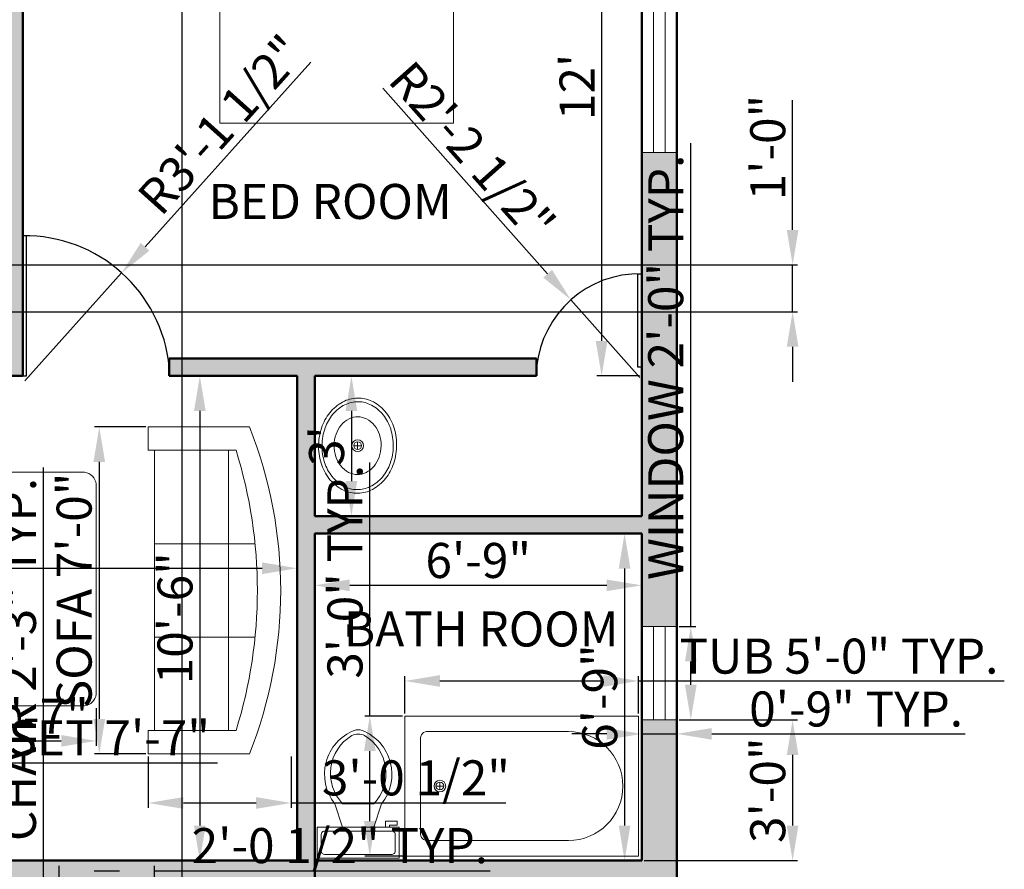
# Model space of a CAD drawing. Units: inches. Extents: x 875413 to 876020, y 447446 to 448210.
# Tile 7 of 8: x 875767 to 876020, y 447795 to 448013. Entities that reach past the tile are written whole.
import ezdxf

# ---------------------------------------------------------------- set-up
doc = ezdxf.new("R2010")
doc.units = ezdxf.units.IN
for name, color, linetype, lineweight in [('A-ANNO-DIMS', 2, 'Continuous', 13), ('A-AREA-IDEN', 7, 'Continuous', 25), ('A-DOOR', 3, 'Continuous', 25), ('A-FLOR-FIXT', 9, 'Continuous', 18), ('A-FURN', 8, 'Continuous', 18), ('A-GLAZ', 4, 'Continuous', 20), ('A-WALL', 7, 'Continuous', 50)]:
    doc.layers.add(name, color=color, linetype=linetype, lineweight=lineweight)
doc.layers.add('A-WALL-PATT', color=18, linetype='Continuous', lineweight=13, true_color=0x000000)
doc.styles.get("Standard").update_dxf_attribs({"font": 'arial.ttf'})
doc.dimstyles.new('ISO-25', dxfattribs={"dimtxt": 9, "dimasz": 9, "dimexe": 1.25, "dimexo": 0.625, "dimtad": 1, "dimdec": 1, "dimrnd": 9, "dimlunit": 3, "dimtxsty": 'Standard', "dimcen": 2.5, "dimadec": 0, "dimazin": 0, "dimtfac": 1, "dimtdec": 1, "dimtmove": 0, "dimatfit": 3, "dimfxl": 1, "dimarcsym": 0})

# ---------------------------------------------------------------- blocks, each defined once
blk = doc.blocks.new('*D6')
at = {"layer": 'A-ANNO-DIMS', "color": 0, "lineweight": -2, "transparency": 16777216}
for p, q in [((875926.08, 448070.02), (875915.14, 448070.02)), ((875916.39, 448061.02), (875916.39, 447930.52)), ((875926.08, 447921.52), (875915.14, 447921.52))]:
    blk.add_line(p, q, dxfattribs=at)
at = {"layer": 'A-ANNO-DIMS', "color": 0, "transparency": 16777216}
for points in [[(875914.89, 448061.02), (875917.89, 448061.02), (875916.39, 448070.02)], [(875914.89, 447930.52), (875917.89, 447930.52), (875916.39, 447921.52)]]:
    blk.add_solid(points, dxfattribs=at)
at = {"layer": 'Defpoints', "color": 0, "transparency": 16777216}
for p in [(875926.7, 448070.02), (875916.39, 447921.52), (875926.7, 447921.52)]:
    blk.add_point(p, dxfattribs=at)
at = {"layer": 'A-ANNO-DIMS', "color": 0, "transparency": 16777216, "insert": (875911.25, 447995.77), "char_height": 9, "attachment_point": 5, "rotation": 90}
blk.add_mtext("12'", dxfattribs=at)
blk = doc.blocks.new('*D10')
at = {"layer": 'A-ANNO-DIMS', "color": 0, "lineweight": -2, "transparency": 16777216}
for p, q in [((875843.33, 447921.52), (875853.37, 447921.52)), ((875852.12, 447912.52), (875852.12, 447894.52)), ((875843.33, 447885.52), (875853.37, 447885.52))]:
    blk.add_line(p, q, dxfattribs=at)
at = {"layer": 'A-ANNO-DIMS', "color": 0, "transparency": 16777216}
for points in [[(875850.62, 447912.52), (875853.62, 447912.52), (875852.12, 447921.52)], [(875850.62, 447894.52), (875853.62, 447894.52), (875852.12, 447885.52)]]:
    blk.add_solid(points, dxfattribs=at)
at = {"layer": 'Defpoints', "color": 0, "transparency": 16777216}
for p in [(875842.7, 447921.52), (875842.7, 447885.52), (875852.12, 447885.52)]:
    blk.add_point(p, dxfattribs=at)
at = {"layer": 'A-ANNO-DIMS', "color": 0, "transparency": 16777216, "insert": (875846.9, 447903.52), "char_height": 9, "attachment_point": 5, "rotation": 90}
blk.add_mtext("3'", dxfattribs=at)
blk = doc.blocks.new('*D11')
at = {"layer": 'A-ANNO-DIMS', "color": 0, "lineweight": -2, "transparency": 16777216}
for p, q in [((875842.7, 447880.39), (875842.7, 447866.47)), ((875926.7, 447880.39), (875926.7, 447866.47)), ((875917.7, 447867.72), (875851.7, 447867.72))]:
    blk.add_line(p, q, dxfattribs=at)
at = {"layer": 'A-ANNO-DIMS', "color": 0, "transparency": 16777216}
for points in [[(875851.7, 447869.22), (875851.7, 447866.22), (875842.7, 447867.72)], [(875917.7, 447869.22), (875917.7, 447866.22), (875926.7, 447867.72)]]:
    blk.add_solid(points, dxfattribs=at)
at = {"layer": 'Defpoints', "color": 0, "transparency": 16777216}
for p in [(875842.7, 447881.02), (875926.7, 447881.02), (875842.7, 447867.72)]:
    blk.add_point(p, dxfattribs=at)
at = {"layer": 'A-ANNO-DIMS', "color": 0, "transparency": 16777216, "insert": (875884.7, 447872.94), "char_height": 9, "attachment_point": 5}
blk.add_mtext('6\'-9"', dxfattribs=at)
blk = doc.blocks.new('*D12')
at = {"layer": 'A-ANNO-DIMS', "color": 0, "lineweight": -2, "transparency": 16777216}
for p, q in [((875926.08, 447881.02), (875921.04, 447881.02)), ((875922.29, 447872.02), (875922.29, 447806.02)), ((875926.08, 447797.02), (875921.04, 447797.02))]:
    blk.add_line(p, q, dxfattribs=at)
at = {"layer": 'A-ANNO-DIMS', "color": 0, "transparency": 16777216}
for points in [[(875920.79, 447872.02), (875923.79, 447872.02), (875922.29, 447881.02)], [(875920.79, 447806.02), (875923.79, 447806.02), (875922.29, 447797.02)]]:
    blk.add_solid(points, dxfattribs=at)
at = {"layer": 'Defpoints', "color": 0, "transparency": 16777216}
for p in [(875926.7, 447881.02), (875922.29, 447797.02), (875926.7, 447797.02)]:
    blk.add_point(p, dxfattribs=at)
at = {"layer": 'A-ANNO-DIMS', "color": 0, "transparency": 16777216, "insert": (875917.07, 447839.02), "char_height": 9, "attachment_point": 5, "rotation": 90}
blk.add_mtext('6\'-9"', dxfattribs=at)
blk = doc.blocks.new('*D13')
at = {"layer": 'A-ANNO-DIMS', "color": 0, "lineweight": -2, "transparency": 16777216}
for p, q in [((875571.2, 447920.89), (875571.2, 447870.86)), ((875838.2, 447920.89), (875838.2, 447870.86)), ((875580.2, 447872.11), (875829.2, 447872.11))]:
    blk.add_line(p, q, dxfattribs=at)
at = {"layer": 'A-ANNO-DIMS', "color": 0, "transparency": 16777216}
for points in [[(875580.2, 447873.61), (875580.2, 447870.61), (875571.2, 447872.11)], [(875829.2, 447873.61), (875829.2, 447870.61), (875838.2, 447872.11)]]:
    blk.add_solid(points, dxfattribs=at)
at = {"layer": 'Defpoints', "color": 0, "transparency": 16777216}
for p in [(875571.2, 447921.52), (875838.2, 447921.52), (875838.2, 447872.11)]:
    blk.add_point(p, dxfattribs=at)
at = {"layer": 'A-ANNO-DIMS', "color": 0, "transparency": 16777216, "insert": (875704.7, 447877.33), "char_height": 9, "attachment_point": 5}
blk.add_mtext('22\'-6"', dxfattribs=at)
blk = doc.blocks.new('*D14')
at = {"layer": 'A-ANNO-DIMS', "color": 0, "lineweight": -2, "transparency": 16777216}
for p, q in [((875837.58, 447921.52), (875811.94, 447921.52)), ((875813.19, 447912.52), (875813.19, 447806.02)), ((875837.58, 447797.02), (875811.94, 447797.02))]:
    blk.add_line(p, q, dxfattribs=at)
at = {"layer": 'A-ANNO-DIMS', "color": 0, "transparency": 16777216}
for points in [[(875811.69, 447912.52), (875814.69, 447912.52), (875813.19, 447921.52)], [(875811.69, 447806.02), (875814.69, 447806.02), (875813.19, 447797.02)]]:
    blk.add_solid(points, dxfattribs=at)
at = {"layer": 'Defpoints', "color": 0, "transparency": 16777216}
for p in [(875838.2, 447921.52), (875813.19, 447797.02), (875838.2, 447797.02)]:
    blk.add_point(p, dxfattribs=at)
at = {"layer": 'A-ANNO-DIMS', "color": 0, "transparency": 16777216, "insert": (875807.97, 447859.27), "char_height": 9, "attachment_point": 5, "rotation": 90}
blk.add_mtext('10\'-6"', dxfattribs=at)
blk = doc.blocks.new('Bed - Queen')
for p, q in [((0, -80.00003), (0, 0)), ((0, 0), (59.99999, 0)), ((59.99999, 0), (59.99999, -80.00003)), ((7.99999, -1.2), (28.79998, -1.2)), ((7.99999, -14.4), (7.99999, -1.2)), ((28.79998, -1.2), (28.79998, -14.4)), ((31.19999, -1.2), (51.99999, -1.2)), ((31.19999, -14.4), (31.19999, -1.2)), ((51.99999, -1.2), (51.99999, -16.4)), ((0, -14.4), (44.8, -14.4)), ((59.99999, -29.6), (44.8, -14.4)), ((44.8, -14.4), (44.8, -29.6)), ((44.8, -16.8), (0, -16.8)), ((51.99999, -16.4), (46.79936, -16.4)), ((44.8, -29.6), (59.99999, -29.6)), ((59.99999, -80.00003), (0, -80.00003))]:
    blk.add_line(p, q)
blk = doc.blocks.new('Sink - Oval top')
for p, q in [((-1, 0), (1, 0)), ((0, 1), (0, -1))]:
    blk.add_line(p, q)
for points in [[(-12.23, 0.39, 0.117634), (-11.46, -3.36, 0.104469), (-8.88, -6.8, 0.090016), (-5.08, -9.07, 0.08192), (-0.32, -10.02, 0.08192), (4.49, -9.38, 0.090016), (8.42, -7.36, 0.104469), (11.22, -4.09, 0.117634), (12.23, -0.39, 0.117634), (11.46, 3.36, 0.104469), (8.88, 6.8, 0.090016), (5.08, 9.07, 0.08192), (0.32, 10.02, 0.08192), (-4.49, 9.38, 0.090016), (-8.42, 7.36, 0.104469), (-11.22, 4.09, 0.117634)], [(-11.29, 0.16, 0.118622), (-10.52, -3.25, 0.104678), (-8.07, -6.36, 0.089562), (-4.54, -8.37, 0.081185), (-0.13, -9.15, 0.081185), (4.3, -8.49, 0.089562), (7.89, -6.58, 0.104678), (10.42, -3.55, 0.118622), (11.29, -0.16, 0.118622), (10.52, 3.25, 0.104678), (8.07, 6.36, 0.089562), (4.54, 8.37, 0.081185), (0.13, 9.15, 0.081185), (-4.3, 8.49, 0.089562), (-7.89, 6.58, 0.104678), (-10.42, 3.55, 0.118622)], [(-7.42, 0.08, 0.118283), (-6.91, -2.17, 0.104607), (-5.29, -4.21, 0.089718), (-2.97, -5.53, 0.081436), (-0.07, -6.04, 0.081436), (2.84, -5.59, 0.089718), (5.2, -4.33, 0.104607), (6.86, -2.32, 0.118283), (7.42, -0.08, 0.118283), (6.91, 2.17, 0.104607), (5.29, 4.21, 0.089718), (2.97, 5.53, 0.081436), (0.07, 6.04, 0.081436), (-2.84, 5.59, 0.089718), (-5.2, 4.33, 0.104607), (-6.86, 2.32, 0.118283)]]:
    blk.add_lwpolyline(points, format="xyb", close=True)
for radius in [1.5, 1]:
    blk.add_circle((0, 0), radius)
blk = doc.blocks.new('Toilet - top')
for p, q in [((9.5, -6), (9.5, -2)), ((-10, -8.5), (-8, -8.5)), ((-10, -9.5), (-10, -8.5)), ((-7, -9.5), (-10, -9.5)), ((-8, -8.5), (-8, -8)), ((-7, -8), (-7, -9.5)), ((-4, -8), (-6, -14)), ((4, -8), (6, -14)), ((4, -14), (-4, -14))]:
    blk.add_line(p, q)
blk.add_lwpolyline([(10.5, -8), (10.5, 0), (-10.5, 0), (-10.5, -8)], close=True)
for points in [[(-9.5, -2), (-9.5, -6)], [(8.5, -1), (-8.5, -1)], [(-8.5, -7), (8.5, -7)]]:
    blk.add_lwpolyline(points)
for centre, radius, start, end in [((-8.62, -1.88), 0.884, 81.8699, 188.1301), ((8.62, -1.88), 0.884, 351.8699, 98.1301), ((-8.62, -6.12), 0.884, 171.8699, 278.1301), ((8.62, -6.12), 0.884, 261.8699, 8.1301), ((3.52, -21.58), 12.17, 141.4691, 247.9714), ((4.2, -21.82), 11.33, 136.3677, 238.9468), ((-3.52, -21.58), 12.17, 292.0284, 38.5307), ((-4.2, -21.82), 11.33, 301.053, 43.6321), ((0, -27.88), 4, 245.7318, 294.2682), ((0, -29), 4, 254.8605, 285.1395)]:
    blk.add_arc(centre, radius, start, end)
blk = doc.blocks.new('Sofa - Roundback 7 ft.')
for p, q in [((-12.00002, -32.4421), (-12.00003, -6.5971)), ((11.99997, -32.4421), (11.99998, -6.5971)), ((-36.000027, -34), (-36.000027, -11.4696)), ((35.99998, -34), (35.99998, -11.4696)), ((-35.999844, -13.3819), (35.9998, -13.3819)), ((-36.000027, -32.4421), (35.99998, -32.4421))]:
    blk.add_line(p, q)
for points in [[(-36.000027, -34), (-42.000027, -34), (-42.000027, -8)], [(41.99998, -8), (41.99998, -34), (35.99998, -34)]]:
    blk.add_lwpolyline(points)
for centre, radius, start, end in [((0, -114.25), 114.25, 68.43141, 111.5686), ((-0.00001, -127.1968), 121.1968, 72.72033, 107.2797)]:
    blk.add_arc(centre, radius, start, end)
blk = doc.blocks.new('Desk - 30 x 60 in.')
for p, q in [((-26.999995, 0), (26.999995, 0)), ((-29.999995, -27), (-29.999995, -3)), ((29.999995, -3), (29.999995, -27)), ((26.999995, -30), (-26.999995, -30)), ((-20.000005, -30), (-20.000005, -31)), ((-16.000005, -31), (-16.000005, -30)), ((15.999995, -31), (15.999995, -30)), ((19.999995, -30), (19.999995, -31)), ((-20.000005, -31), (-16.000005, -31)), ((19.999995, -31), (15.999995, -31))]:
    blk.add_line(p, q)
for centre, start, end in [((-26.499995, -3.5), 98.1301, 171.8699), ((26.499995, -3.5), 8.130102, 81.8699), ((-26.499995, -26.5), 188.1301, 261.8699), ((26.499995, -26.5), 278.1301, 351.8699)]:
    blk.add_arc(centre, 3.535534, start, end)
blk = doc.blocks.new('Bath Tub - 26 x 60 in.')
for p, q in [((9, -17), (9, -19)), ((8, -18), (10, -18))]:
    blk.add_line(p, q)
blk.add_lwpolyline([(0, -36), (0, 0), (60, 0), (60, -36)], close=True)
for points in [[(6, -4), (42, -4)], [(4, -30), (4, -6)], [(42, -32), (6, -32)]]:
    blk.add_lwpolyline(points)
for radius in [1.5, 1]:
    blk.add_circle((9, -18), radius)
for centre, radius, start, end in [((5.75, -5.75), 1.77, 81.8699, 188.1301), ((42, -18), 14, 270, 90), ((5.75, -30.25), 1.77, 171.8699, 278.1301)]:
    blk.add_arc(centre, radius, start, end)
blk = doc.blocks.new('WIN-60IN')
for p, q in [((0, 9), (0, 0)), ((60, 9), (60, 0)), ((60, 6), (0, 6)), ((60, 3), (0, 3))]:
    blk.add_line(p, q)
blk = doc.blocks.new('WIN-24IN')
for p, q in [((0, 24), (9, 24)), ((3, 0), (3, 24)), ((6, 0), (6, 24)), ((0, 0), (9, 0))]:
    blk.add_line(p, q)
blk = doc.blocks.new('*D43')
at = {"layer": 'A-ANNO-DIMS', "color": 0, "lineweight": -2, "transparency": 16777216}
for p, q in [((875939.3, 447857.16), (875939.3, 447981.3)), ((875936.33, 447857.16), (875940.55, 447857.16)), ((875939.3, 447842.16), (875939.3, 447848.16)), ((875936.33, 447833.16), (875940.55, 447833.16))]:
    blk.add_line(p, q, dxfattribs=at)
at = {"layer": 'A-ANNO-DIMS', "color": 0, "transparency": 16777216}
for points in [[(875937.8, 447848.16), (875940.8, 447848.16), (875939.3, 447857.16)], [(875937.8, 447842.16), (875940.8, 447842.16), (875939.3, 447833.16)]]:
    blk.add_solid(points, dxfattribs=at)
at = {"layer": 'Defpoints', "color": 0, "transparency": 16777216}
for p in [(875935.7, 447857.16), (875939.3, 447857.16), (875935.7, 447833.16)]:
    blk.add_point(p, dxfattribs=at)
at = {"layer": 'A-ANNO-DIMS', "color": 0, "transparency": 16777216, "insert": (875934.02, 447923.73), "char_height": 9, "attachment_point": 5, "rotation": 90}
blk.add_mtext('WINDOW 2\'-0" TYP.', dxfattribs=at)
blk = doc.blocks.new('*D44')
at = {"layer": 'A-ANNO-DIMS', "color": 0, "lineweight": -2, "transparency": 16777216}
for p, q in [((875926.7, 447832.54), (875926.7, 447828.31)), ((875935.7, 447832.54), (875935.7, 447828.31)), ((875917.7, 447829.56), (875908.7, 447829.56)), ((875926.7, 447829.56), (875935.7, 447829.56)), ((875944.7, 447829.56), (876009.81, 447829.56))]:
    blk.add_line(p, q, dxfattribs=at)
at = {"layer": 'A-ANNO-DIMS', "color": 0, "transparency": 16777216}
for points in [[(875917.7, 447831.06), (875917.7, 447828.06), (875926.7, 447829.56)], [(875944.7, 447831.06), (875944.7, 447828.06), (875935.7, 447829.56)]]:
    blk.add_solid(points, dxfattribs=at)
at = {"layer": 'Defpoints', "color": 0, "transparency": 16777216}
for p in [(875926.7, 447833.16), (875935.7, 447833.16), (875935.7, 447829.56)]:
    blk.add_point(p, dxfattribs=at)
at = {"layer": 'A-ANNO-DIMS', "color": 0, "transparency": 16777216, "insert": (875981.76, 447834.78), "char_height": 9, "attachment_point": 5}
blk.add_mtext('0\'-9" TYP.', dxfattribs=at)
blk = doc.blocks.new('*D51')
at = {"layer": 'A-ANNO-DIMS', "color": 0, "lineweight": -2, "transparency": 16777216}
for p, q in [((875865.85, 447834.78), (875865.85, 447844.4)), ((875874.85, 447843.15), (875916.85, 447843.15)), ((875925.85, 447834.78), (875925.85, 447844.4)), ((875925.85, 447843.15), (876019.83, 447843.15))]:
    blk.add_line(p, q, dxfattribs=at)
at = {"layer": 'A-ANNO-DIMS', "color": 0, "transparency": 16777216}
for points in [[(875874.85, 447844.65), (875874.85, 447841.65), (875865.85, 447843.15)], [(875916.85, 447844.65), (875916.85, 447841.65), (875925.85, 447843.15)]]:
    blk.add_solid(points, dxfattribs=at)
at = {"layer": 'Defpoints', "color": 0, "transparency": 16777216}
for p in [(875925.85, 447843.15), (875865.85, 447834.15), (875925.85, 447834.15)]:
    blk.add_point(p, dxfattribs=at)
at = {"layer": 'A-ANNO-DIMS', "color": 0, "transparency": 16777216, "insert": (875977.34, 447848.37), "char_height": 9, "attachment_point": 5}
blk.add_mtext('TUB 5\'-0" TYP.', dxfattribs=at)
blk = doc.blocks.new('*D52')
at = {"layer": 'A-ANNO-DIMS', "color": 0, "lineweight": -2, "transparency": 16777216}
for p, q in [((875856.85, 447834.15), (875856.85, 447899.26)), ((875865.23, 447834.15), (875855.6, 447834.15)), ((875856.85, 447807.15), (875856.85, 447825.15)), ((875865.23, 447798.15), (875855.6, 447798.15))]:
    blk.add_line(p, q, dxfattribs=at)
at = {"layer": 'A-ANNO-DIMS', "color": 0, "transparency": 16777216}
for points in [[(875855.35, 447825.15), (875858.35, 447825.15), (875856.85, 447834.15)], [(875855.35, 447807.15), (875858.35, 447807.15), (875856.85, 447798.15)]]:
    blk.add_solid(points, dxfattribs=at)
at = {"layer": 'Defpoints', "color": 0, "transparency": 16777216}
for p in [(875856.85, 447834.15), (875865.85, 447834.15), (875865.85, 447798.15)]:
    blk.add_point(p, dxfattribs=at)
at = {"layer": 'A-ANNO-DIMS', "color": 0, "transparency": 16777216, "insert": (875851.63, 447871.2), "char_height": 9, "attachment_point": 5, "rotation": 90}
blk.add_mtext('3\'-0" TYP.', dxfattribs=at)
blk = doc.blocks.new('*D53')
at = {"layer": 'A-ANNO-DIMS', "color": 0, "lineweight": -2, "transparency": 16777216}
for p, q in [((875617.53, 447835.12), (875617.53, 447820.85)), ((875708.53, 447835.12), (875708.53, 447820.85)), ((875626.53, 447822.1), (875699.53, 447822.1)), ((875708.53, 447822.1), (875817.7, 447822.1))]:
    blk.add_line(p, q, dxfattribs=at)
at = {"layer": 'A-ANNO-DIMS', "color": 0, "transparency": 16777216}
for points in [[(875626.53, 447823.6), (875626.53, 447820.6), (875617.53, 447822.1)], [(875699.53, 447823.6), (875699.53, 447820.6), (875708.53, 447822.1)]]:
    blk.add_solid(points, dxfattribs=at)
at = {"layer": 'Defpoints', "color": 0, "transparency": 16777216}
for p in [(875617.53, 447835.75), (875708.53, 447835.75), (875708.53, 447822.1)]:
    blk.add_point(p, dxfattribs=at)
at = {"layer": 'A-ANNO-DIMS', "color": 0, "transparency": 16777216, "insert": (875767.62, 447827.38), "char_height": 9, "attachment_point": 5}
blk.add_mtext('DINING SET 7\'-7"', dxfattribs=at)
blk = doc.blocks.new('*D57')
at = {"layer": 'A-ANNO-DIMS', "color": 0, "lineweight": -2, "transparency": 16777216}
for p, q in [((875773.04, 447790.36), (875773.04, 447897.98)), ((875776.46, 447790.36), (875771.79, 447790.36)), ((875773.04, 447772.36), (875773.04, 447781.36)), ((875776.46, 447763.36), (875771.79, 447763.36))]:
    blk.add_line(p, q, dxfattribs=at)
at = {"layer": 'A-ANNO-DIMS', "color": 0, "transparency": 16777216}
for points in [[(875771.54, 447781.36), (875774.54, 447781.36), (875773.04, 447790.36)], [(875771.54, 447772.36), (875774.54, 447772.36), (875773.04, 447763.36)]]:
    blk.add_solid(points, dxfattribs=at)
at = {"layer": 'Defpoints', "color": 0, "transparency": 16777216}
for p in [(875773.04, 447790.36), (875777.09, 447790.36), (875777.09, 447763.36)]:
    blk.add_point(p, dxfattribs=at)
at = {"layer": 'A-ANNO-DIMS', "color": 0, "transparency": 16777216, "insert": (875767.76, 447848.67), "char_height": 9, "attachment_point": 5, "rotation": 90}
blk.add_mtext('CHAIR 2\'-3" TYP.', dxfattribs=at)
blk = doc.blocks.new('*D58')
at = {"layer": 'A-ANNO-DIMS', "color": 0, "lineweight": -2, "transparency": 16777216}
for p, q in [((875777.09, 447790.98), (875777.09, 447795.66)), ((875801.52, 447790.98), (875801.52, 447795.66)), ((875786.09, 447794.41), (875792.52, 447794.41)), ((875801.52, 447794.41), (875887.76, 447794.41))]:
    blk.add_line(p, q, dxfattribs=at)
at = {"layer": 'A-ANNO-DIMS', "color": 0, "transparency": 16777216}
for points in [[(875786.09, 447795.91), (875786.09, 447792.91), (875777.09, 447794.41)], [(875792.52, 447795.91), (875792.52, 447792.91), (875801.52, 447794.41)]]:
    blk.add_solid(points, dxfattribs=at)
at = {"layer": 'Defpoints', "color": 0, "transparency": 16777216}
for p in [(875801.52, 447794.41), (875777.09, 447790.36), (875801.52, 447790.36)]:
    blk.add_point(p, dxfattribs=at)
at = {"layer": 'A-ANNO-DIMS', "color": 0, "transparency": 16777216, "insert": (875849.14, 447799.69), "char_height": 9, "attachment_point": 5}
blk.add_mtext('2\'-0 1/2" TYP.', dxfattribs=at)
blk = doc.blocks.new('*D59')
at = {"layer": 'A-ANNO-DIMS', "color": 0, "lineweight": -2, "transparency": 16777216}
for p, q in [((875799.33, 447908.41), (875786.11, 447908.41)), ((875787.36, 447899.41), (875787.36, 447833.41)), ((875799.33, 447824.41), (875786.11, 447824.41))]:
    blk.add_line(p, q, dxfattribs=at)
at = {"layer": 'A-ANNO-DIMS', "color": 0, "transparency": 16777216}
for points in [[(875785.86, 447899.41), (875788.86, 447899.41), (875787.36, 447908.41)], [(875785.86, 447833.41), (875788.86, 447833.41), (875787.36, 447824.41)]]:
    blk.add_solid(points, dxfattribs=at)
at = {"layer": 'Defpoints', "color": 0, "transparency": 16777216}
for p in [(875799.96, 447908.41), (875787.36, 447824.41), (875799.96, 447824.41)]:
    blk.add_point(p, dxfattribs=at)
at = {"layer": 'A-ANNO-DIMS', "color": 0, "transparency": 16777216, "insert": (875782.07, 447866.41), "char_height": 9, "attachment_point": 5, "rotation": 90}
blk.add_mtext('SOFA 7\'-0"', dxfattribs=at)
blk = doc.blocks.new('*D60')
at = {"layer": 'A-ANNO-DIMS', "color": 0, "lineweight": -2, "transparency": 16777216}
for p, q in [((875799.96, 447823.78), (875799.96, 447810.56)), ((875836.62, 447823.78), (875836.62, 447810.56)), ((875808.96, 447811.81), (875827.62, 447811.81)), ((875836.62, 447811.81), (875891.76, 447811.81))]:
    blk.add_line(p, q, dxfattribs=at)
at = {"layer": 'A-ANNO-DIMS', "color": 0, "transparency": 16777216}
for points in [[(875808.96, 447813.31), (875808.96, 447810.31), (875799.96, 447811.81)], [(875827.62, 447813.31), (875827.62, 447810.31), (875836.62, 447811.81)]]:
    blk.add_solid(points, dxfattribs=at)
at = {"layer": 'Defpoints', "color": 0, "transparency": 16777216}
for p in [(875799.96, 447824.41), (875836.62, 447824.41), (875836.62, 447811.81)]:
    blk.add_point(p, dxfattribs=at)
at = {"layer": 'A-ANNO-DIMS', "color": 0, "transparency": 16777216, "insert": (875868.69, 447817.09), "char_height": 9, "attachment_point": 5}
blk.add_mtext('3\'-0 1/2"', dxfattribs=at)
blk = doc.blocks.new('*D62')
at = {"layer": 'A-ANNO-DIMS', "color": 0, "lineweight": -2, "transparency": 16777216}
for p, q in [((875755.58, 447836.14), (875755.58, 447826.52)), ((875786.58, 447836.14), (875786.58, 447826.52)), ((875764.58, 447827.77), (875777.58, 447827.77))]:
    blk.add_line(p, q, dxfattribs=at)
at = {"layer": 'A-ANNO-DIMS', "color": 0, "transparency": 16777216}
for points in [[(875764.58, 447829.27), (875764.58, 447826.27), (875755.58, 447827.77)], [(875777.58, 447829.27), (875777.58, 447826.27), (875786.58, 447827.77)]]:
    blk.add_solid(points, dxfattribs=at)
at = {"layer": 'Defpoints', "color": 0, "transparency": 16777216}
for p in [(875755.58, 447836.77), (875786.58, 447836.77), (875786.58, 447827.77)]:
    blk.add_point(p, dxfattribs=at)
at = {"layer": 'A-ANNO-DIMS', "color": 0, "transparency": 16777216, "insert": (875771.08, 447832.91), "char_height": 9, "attachment_point": 5}
blk.add_mtext('2\'-7"', dxfattribs=at)
blk = doc.blocks.new('*D75')
at = {"layer": 'A-ANNO-DIMS', "color": 0, "lineweight": -2, "transparency": 16777216}
for p, q in [((875936.33, 447833.16), (875966.7, 447833.16)), ((875965.45, 447824.16), (875965.45, 447806.02)), ((875927.33, 447797.02), (875966.7, 447797.02))]:
    blk.add_line(p, q, dxfattribs=at)
at = {"layer": 'A-ANNO-DIMS', "color": 0, "transparency": 16777216}
for points in [[(875963.95, 447824.16), (875966.95, 447824.16), (875965.45, 447833.16)], [(875963.95, 447806.02), (875966.95, 447806.02), (875965.45, 447797.02)]]:
    blk.add_solid(points, dxfattribs=at)
at = {"layer": 'Defpoints', "color": 0, "transparency": 16777216}
for p in [(875935.7, 447833.16), (875926.7, 447797.02), (875965.45, 447797.02)]:
    blk.add_point(p, dxfattribs=at)
at = {"layer": 'A-ANNO-DIMS', "color": 0, "transparency": 16777216, "insert": (875960.23, 447815.09), "char_height": 9, "attachment_point": 5, "rotation": 90}
blk.add_mtext('3\'-0"', dxfattribs=at)
blk = doc.blocks.new('*D78')
at = {"layer": 'A-ANNO-DIMS', "color": 0, "lineweight": -2, "transparency": 16777216}
for p, q in [((875965.45, 447959.02), (875965.45, 447992.34)), ((875763.83, 447950.02), (875966.7, 447950.02)), ((875965.45, 447938.02), (875965.45, 447950.02)), ((875763.83, 447938.02), (875966.7, 447938.02)), ((875965.45, 447929.02), (875965.45, 447920.02))]:
    blk.add_line(p, q, dxfattribs=at)
at = {"layer": 'A-ANNO-DIMS', "color": 0, "transparency": 16777216}
for points in [[(875963.95, 447959.02), (875966.95, 447959.02), (875965.45, 447950.02)], [(875963.95, 447929.02), (875966.95, 447929.02), (875965.45, 447938.02)]]:
    blk.add_solid(points, dxfattribs=at)
at = {"layer": 'Defpoints', "color": 0, "transparency": 16777216}
for p in [(875763.2, 447950.02), (875965.45, 447950.02), (875763.2, 447938.02)]:
    blk.add_point(p, dxfattribs=at)
at = {"layer": 'A-ANNO-DIMS', "color": 0, "transparency": 16777216, "insert": (875960.23, 447980.18), "char_height": 9, "attachment_point": 5, "rotation": 90}
blk.add_mtext('1\'-0"', dxfattribs=at)
blk = doc.blocks.new('*D80')
at = {"layer": 'A-ANNO-DIMS', "color": 0, "lineweight": -2, "transparency": 16777216}
for p, q in [((875748.63, 447673.14), (875748.63, 448110.02)), ((875757.63, 448108.77), (875799.63, 448108.77)), ((875808.63, 447673.14), (875808.63, 448110.02))]:
    blk.add_line(p, q, dxfattribs=at)
at = {"layer": 'A-ANNO-DIMS', "color": 0, "transparency": 16777216}
for points in [[(875757.63, 448110.27), (875757.63, 448107.27), (875748.63, 448108.77)], [(875799.63, 448110.27), (875799.63, 448107.27), (875808.63, 448108.77)]]:
    blk.add_solid(points, dxfattribs=at)
at = {"layer": 'Defpoints', "color": 0, "transparency": 16777216}
for p in [(875808.63, 448108.77), (875748.63, 447672.52), (875808.63, 447672.52)]:
    blk.add_point(p, dxfattribs=at)
at = {"layer": 'A-ANNO-DIMS', "color": 0, "transparency": 16777216, "insert": (875778.63, 448113.99), "char_height": 9, "attachment_point": 5}
blk.add_mtext('5\'-0"', dxfattribs=at)
blk = doc.blocks.new('*D94')
at = {"layer": 'A-ANNO-DIMS', "color": 0, "lineweight": -2, "transparency": 16777216}
for p, q in [((875841.68, 448002.16), (875799.12, 447954.69)), ((875768.2, 447920.22), (875793.11, 447947.99))]:
    blk.add_line(p, q, dxfattribs=at)
at = {"layer": 'A-ANNO-DIMS', "color": 0, "transparency": 16777216}
blk.add_solid([(875798, 447955.69), (875800.23, 447953.69), (875793.11, 447947.99)], dxfattribs=at)
at = {"layer": 'Defpoints', "color": 0, "transparency": 16777216}
for p in [(875793.11, 447947.99), (875768.2, 447920.22)]:
    blk.add_point(p, dxfattribs=at)
at = {"layer": 'A-ANNO-DIMS', "color": 0, "transparency": 16777216, "insert": (875819.47, 447985.3), "char_height": 9, "attachment_point": 5, "rotation": 48.1157}
blk.add_mtext('R3\'-1 1/2"', dxfattribs=at)
blk = doc.blocks.new('*D100')
at = {"layer": 'A-ANNO-DIMS', "color": 0, "lineweight": -2, "transparency": 16777216}
for p, q in [((875860.18, 447995.43), (875902.53, 447947.77)), ((875926.2, 447921.14), (875908.51, 447941.05))]:
    blk.add_line(p, q, dxfattribs=at)
at = {"layer": 'A-ANNO-DIMS', "color": 0, "transparency": 16777216}
blk.add_solid([(875903.65, 447948.77), (875901.41, 447946.78), (875908.51, 447941.05)], dxfattribs=at)
at = {"layer": 'Defpoints', "color": 0, "transparency": 16777216}
for p in [(875908.51, 447941.05), (875926.2, 447921.14)]:
    blk.add_point(p, dxfattribs=at)
at = {"layer": 'A-ANNO-DIMS', "color": 0, "transparency": 16777216, "insert": (875882.31, 447978.47), "char_height": 9, "attachment_point": 5, "rotation": 311.6278}
blk.add_mtext('R2\'-2 1/2"', dxfattribs=at)

msp = doc.modelspace()

# ---------------------------------------------------------------- hatches: boundary and pattern name
at = {"layer": 'A-WALL-PATT'}
h = msp.add_hatch(color=256, dxfattribs=at)
h.dxf.hatch_style = 1
h.paths.add_polyline_path([(875470.7, 447985.13), (875461.7, 447985.13), (875461.7, 447865.29), (875470.7, 447865.29), (875470.7, 447881.02), (875566.7, 447881.02), (875566.7, 447797.02), (875571.2, 447797.02), (875571.2, 447885.52), (875571.2, 447921.52), (875603.29, 447921.52), (875603.29, 447926.02), (875501.27, 447926.02), (875501.27, 447921.52), (875566.7, 447921.52), (875566.7, 447885.52), (875470.7, 447885.52), (875470.7, 447921.52), (875470.7, 447926.02)])
h.paths.add_polyline_path([(875470.7, 448070.02), (875518.96, 448070.02), (875518.96, 448079.02), (875461.7, 448079.02), (875461.7, 448045.13), (875470.7, 448045.13)])
h.paths.add_polyline_path([(875819.9, 448079.02), (875578.96, 448079.02), (875578.96, 448070.02), (875638.7, 448070.02), (875638.7, 447921.52), (875643.2, 447921.52), (875643.2, 448070.02), (875763.2, 448070.02), (875763.2, 447921.52), (875767.7, 447921.52), (875767.7, 448070.02), (875819.9, 448070.02)])
h.paths.add_polyline_path([(875935.7, 447978.92), (875926.7, 447978.92), (875926.7, 447926.02), (875926.7, 447921.52), (875926.7, 447885.52), (875842.7, 447885.52), (875842.7, 447921.52), (875899.7, 447921.52), (875899.7, 447926.02), (875805.34, 447926.02), (875805.34, 447921.52), (875838.2, 447921.52), (875838.2, 447885.52), (875838.2, 447797.02), (875689.7, 447797.02), (875689.7, 447792.52), (875842.7, 447792.52), (875842.7, 447881.02), (875926.7, 447881.02), (875926.7, 447857.16), (875935.7, 447857.16)])
h.paths.add_polyline_path([(875935.7, 448079.02), (875879.9, 448079.02), (875879.9, 448070.02), (875926.7, 448070.02), (875926.7, 448038.92), (875935.7, 448038.92)])
h.paths.add_polyline_path([(875935.7, 447833.16), (875926.7, 447833.16), (875926.7, 447797.02), (875842.7, 447797.02), (875842.7, 447792.52), (875926.7, 447792.52), (875926.7, 447756.52), (875935.7, 447756.52)])
h.paths.add_polyline_path([(875935.7, 447732.52), (875926.7, 447732.52), (875926.7, 447692.75, -0.007222), (875926.81, 447692.41, -0.08192), (875927.45, 447687.6, -0.071798), (875926.7, 447683.4), (875926.7, 447672.52), (875808.63, 447672.52), (875808.63, 447668.02), (875926.7, 447668.02), (875926.7, 447663.19), (875935.7, 447663.19)])
h.paths.add_polyline_path([(875842.7, 447792.52), (875838.2, 447792.52), (875838.2, 447704.02), (875842.7, 447704.02)])
h.paths.add_polyline_path([(875470.7, 447792.52), (875619.2, 447792.52), (875619.2, 447797.02), (875470.7, 447797.02), (875470.7, 447841.29), (875461.7, 447841.29), (875461.7, 447764.71), (875470.7, 447764.71)])
h.paths.add_polyline_path([(875619.2, 447760.51), (875616.95, 447760.51, -0.018388), (875614.7, 447760.37), (875614.7, 447672.52), (875470.7, 447672.52), (875470.7, 447704.71), (875461.7, 447704.71), (875461.7, 447640.7), (875470.7, 447640.7), (875470.7, 447668.02), (875619.2, 447668.02)])
h.paths.add_polyline_path([(875511.12, 447554.02), (875470.7, 447554.02), (875470.7, 447580.7), (875461.7, 447580.7), (875461.7, 447545.02), (875511.12, 447545.02)])
h.paths.add_polyline_path([(875656.47, 447554.02), (875620.05, 447554.02, -0.057036), (875616.67, 447553.74, -0.040891), (875614.26, 447554.02), (875571.12, 447554.02), (875571.12, 447545.02), (875656.47, 447545.02)])
h.paths.add_polyline_path([(875643.2, 447613.27), (875685.21, 447613.27), (875685.21, 447617.77), (875685.21, 447623.8), (875680.71, 447623.8), (875680.71, 447617.77), (875618.23, 447617.77), (875618.23, 447623.8), (875613.73, 447623.8), (875613.73, 447617.77), (875613.73, 447613.27), (875638.7, 447613.27), (875638.7, 447554.02), (875643.2, 447554.02)])
h.paths.add_polyline_path([(875694.2, 447760.28), (875689.7, 447760.28), (875689.7, 447668.02), (875748.63, 447668.02), (875748.63, 447672.52), (875694.2, 447672.52)])

# ---------------------------------------------------------------- linework, layer by layer
at = {"layer": 'A-DOOR'}
for p, q in [((875768.7, 447957.52), (875767.7, 447957.52)), ((875768.7, 447921.52), (875768.7, 447957.52)), ((875925.7, 447923.77), (875925.7, 447947.77)), ((875925.7, 447947.77), (875926.7, 447947.77)), ((875926.7, 447923.77), (875925.7, 447923.77)), ((875767.7, 447921.52), (875768.7, 447921.52))]:
    msp.add_line(p, q, dxfattribs=at)
for centre, radius, start, end in [((875768.2, 447920.22), 37.31, 5.4633, 90.768), ((875926.2, 447921.14), 26.64, 88.9244, 174.3318)]:
    msp.add_arc(centre, radius, start, end, dxfattribs=at)
at = {"layer": 'A-WALL'}
for p, q in [((875935.7, 447663.19), (875935.7, 448079.02)), ((875767.7, 448070.02), (875767.7, 447921.52)), ((875926.7, 447926.02), (875926.7, 448070.02)), ((875899.7, 447926.02), (875805.34, 447926.02)), ((875805.34, 447926.02), (875805.34, 447921.52)), ((875899.7, 447926.02), (875899.7, 447921.52)), ((875926.7, 447926.02), (875926.7, 447921.52)), ((875763.2, 447921.52), (875767.7, 447921.52)), ((875838.2, 447921.52), (875805.34, 447921.52)), ((875838.2, 447885.52), (875838.2, 447921.52)), ((875899.7, 447921.52), (875842.7, 447921.52)), ((875842.7, 447885.52), (875842.7, 447921.52)), ((875926.7, 447885.52), (875926.7, 447921.52)), ((875838.2, 447797.02), (875838.2, 447885.52)), ((875926.7, 447885.52), (875842.7, 447885.52)), ((875926.7, 447881.02), (875842.7, 447881.02)), ((875842.7, 447704.02), (875842.7, 447881.02)), ((875926.7, 447797.02), (875926.7, 447881.02)), ((875838.2, 447797.02), (875689.7, 447797.02)), ((875926.7, 447797.02), (875842.7, 447797.02))]:
    msp.add_line(p, q, dxfattribs=at)

# ---------------------------------------------------------------- block references
at = {"layer": 'A-FLOR-FIXT'}
for name, p, rotation in [('Sink - Oval top', (875853.72, 447903.6), 270), ('Toilet - top', (875853.87, 447797.6), 180)]:
    msp.add_blockref(name, p, dxfattribs=dict(at, rotation=rotation))
msp.add_blockref('Bath Tub - 26 x 60 in.', (875865.85, 447834.15), dxfattribs=at)
at = {"layer": 'A-FURN'}
msp.add_blockref('Bed - Queen', (875818.33, 448066.46), dxfattribs=at)
at = {"layer": 'A-FURN', "rotation": 270}
for name, p in [('Sofa - Roundback 7 ft.', (875833.96, 447866.41)), ('Desk - 30 x 60 in.', (875786.58, 447866.77))]:
    msp.add_blockref(name, p, dxfattribs=at)
at = {"layer": 'A-GLAZ', "rotation": 269.9999999998151}
msp.add_blockref('WIN-60IN', (875926.7, 448038.92), dxfattribs=at)
at = {"layer": 'A-GLAZ'}
msp.add_blockref('WIN-24IN', (875926.7, 447833.16), dxfattribs=at)

# ---------------------------------------------------------------- texts
at = {"layer": 'A-AREA-IDEN', "char_height": 9, "attachment_point": 1}
for s, insert in [('BED ROOM', (875815.41, 447970.84)), ('BATH ROOM', (875850.17, 447861.01))]:
    msp.add_mtext_dynamic_manual_height_columns(s, width=100.7812, gutter_width=12.5, heights=[0], dxfattribs=dict(at, insert=insert))

# ---------------------------------------------------------------- dimensions: what is measured, and where the dimension line sits
at = {"layer": 'A-ANNO-DIMS'}
for base, p1, p2, override, picture, middle in [((875808.63, 448108.77), (875748.63, 447672.52), (875808.63, 447672.52), {"dimdec": 1, "dimlfac": 1, "dimrnd": 0, "dimzin": 1, "dimdsep": 46, "dimlunit": 4, "dimfrac": 2}, '*D80', (875778.63, 448113.99)), ((875838.2, 447872.11), (875571.2, 447921.52), (875838.2, 447921.52), {"dimclrd": 0, "dimclre": 0, "dimclrt": 0}, '*D13', (875704.7, 447877.33)), ((875842.7, 447867.72), (875926.7, 447881.02), (875842.7, 447881.02), {"dimclrd": 0, "dimclre": 0, "dimclrt": 0}, '*D11', (875884.7, 447872.94)), ((875786.58, 447827.77), (875755.58, 447836.77), (875786.58, 447836.77), {"dimdec": 1, "dimlfac": 1, "dimrnd": 0, "dimzin": 1, "dimdsep": 46, "dimlunit": 4, "dimfrac": 2}, '*D62', (875771.08, 447832.91)), ((875836.62, 447811.81), (875799.96, 447824.41), (875836.62, 447824.41), {"dimdec": 1, "dimlfac": 1, "dimrnd": 0, "dimzin": 1, "dimdsep": 46, "dimlunit": 4, "dimfrac": 2}, '*D60', (875868.69, 447817.09))]:
    dim = msp.add_linear_dim(base=base, p1=p1, p2=p2, dimstyle='ISO-25', override=override, dxfattribs=at)
    dim.commit()
    dim.dimension.update_dxf_attribs({"geometry": picture, "text_midpoint": middle})
for base, p1, p2, override, picture, middle in [((875916.39, 447921.52), (875926.7, 448070.02), (875926.7, 447921.52), {"dimclrd": 0, "dimclre": 0, "dimclrt": 0}, '*D6', (875911.25, 447995.77)), ((875965.45, 447950.02), (875763.2, 447938.02), (875763.2, 447950.02), {"dimdec": 1, "dimlfac": 1, "dimrnd": 0, "dimzin": 1, "dimdsep": 46, "dimlunit": 4, "dimfrac": 2}, '*D78', (875960.23, 447980.18)), ((875813.19, 447797.02), (875838.2, 447921.52), (875838.2, 447797.02), {"dimclrd": 0, "dimclre": 0, "dimclrt": 0}, '*D14', (875807.97, 447859.27)), ((875852.12, 447885.52), (875842.7, 447921.52), (875842.7, 447885.52), {"dimclrd": 0, "dimclre": 0, "dimclrt": 0}, '*D10', (875846.9, 447903.52)), ((875922.29, 447797.02), (875926.7, 447881.02), (875926.7, 447797.02), {"dimclrd": 0, "dimclre": 0, "dimclrt": 0}, '*D12', (875917.07, 447839.02)), ((875965.45, 447797.02), (875935.7, 447833.16), (875926.7, 447797.02), {"dimdec": 1, "dimlfac": 1, "dimrnd": 0, "dimzin": 1, "dimdsep": 46, "dimlunit": 4, "dimfrac": 2}, '*D75', (875960.23, 447815.09))]:
    dim = msp.add_linear_dim(base=base, p1=p1, p2=p2, angle=90, dimstyle='ISO-25', override=override, dxfattribs=at)
    dim.commit()
    dim.dimension.update_dxf_attribs({"geometry": picture, "text_midpoint": middle})
for center, mpoint, picture, middle in [((875768.2, 447920.22), (875793.11, 447947.99), '*D94', (875819.47, 447985.3)), ((875926.2, 447921.14), (875908.51, 447941.05), '*D100', (875882.31, 447978.47))]:
    dim = msp.add_radius_dim(center=center, mpoint=mpoint, dimstyle='ISO-25', override={"dimdec": 1, "dimlfac": 1, "dimrnd": 0, "dimzin": 1, "dimdsep": 46, "dimlunit": 4, "dimfrac": 2}, dxfattribs=at)
    dim.commit()
    dim.dimension.update_dxf_attribs({"geometry": picture, "text_midpoint": middle})
for base, p1, p2, angle, text, picture, middle in [((875939.3, 447857.16), (875935.7, 447833.16), (875935.7, 447857.16), 90, 'WINDOW <> TYP.', '*D43', (875934.02, 447923.73)), ((875787.36, 447824.41), (875799.96, 447908.41), (875799.96, 447824.41), 270, 'SOFA <>', '*D59', (875782.07, 447866.41)), ((875856.85, 447834.15), (875865.85, 447798.15), (875865.85, 447834.15), 90, '<> TYP.', '*D52', (875851.63, 447871.2)), ((875773.04, 447790.36), (875777.09, 447763.36), (875777.09, 447790.36), 90, 'CHAIR <> TYP.', '*D57', (875767.76, 447848.67))]:
    dim = msp.add_linear_dim(base=base, p1=p1, p2=p2, angle=angle, text=text, dimstyle='ISO-25', override={"dimdec": 1, "dimlfac": 1, "dimrnd": 0, "dimzin": 1, "dimdsep": 46, "dimlunit": 4, "dimfrac": 2}, dxfattribs=at)
    dim.commit()
    dim.dimension.update_dxf_attribs({"geometry": picture, "text_midpoint": middle})
for base, p1, p2, text, picture, middle in [((875925.85, 447843.15), (875865.85, 447834.15), (875925.85, 447834.15), 'TUB <> TYP.', '*D51', (875977.34, 447848.37)), ((875708.53, 447822.1), (875617.53, 447835.75), (875708.53, 447835.75), 'DINING SET <>', '*D53', (875767.62, 447827.38)), ((875935.7, 447829.56), (875926.7, 447833.16), (875935.7, 447833.16), '<> TYP.', '*D44', (875981.76, 447834.78)), ((875801.52, 447794.41), (875777.09, 447790.36), (875801.52, 447790.36), '<> TYP.', '*D58', (875849.14, 447799.69))]:
    dim = msp.add_linear_dim(base=base, p1=p1, p2=p2, text=text, dimstyle='ISO-25', override={"dimdec": 1, "dimlfac": 1, "dimrnd": 0, "dimzin": 1, "dimdsep": 46, "dimlunit": 4, "dimfrac": 2}, dxfattribs=at)
    dim.commit()
    dim.dimension.update_dxf_attribs({"geometry": picture, "text_midpoint": middle})

doc.saveas('drawing.dxf')
